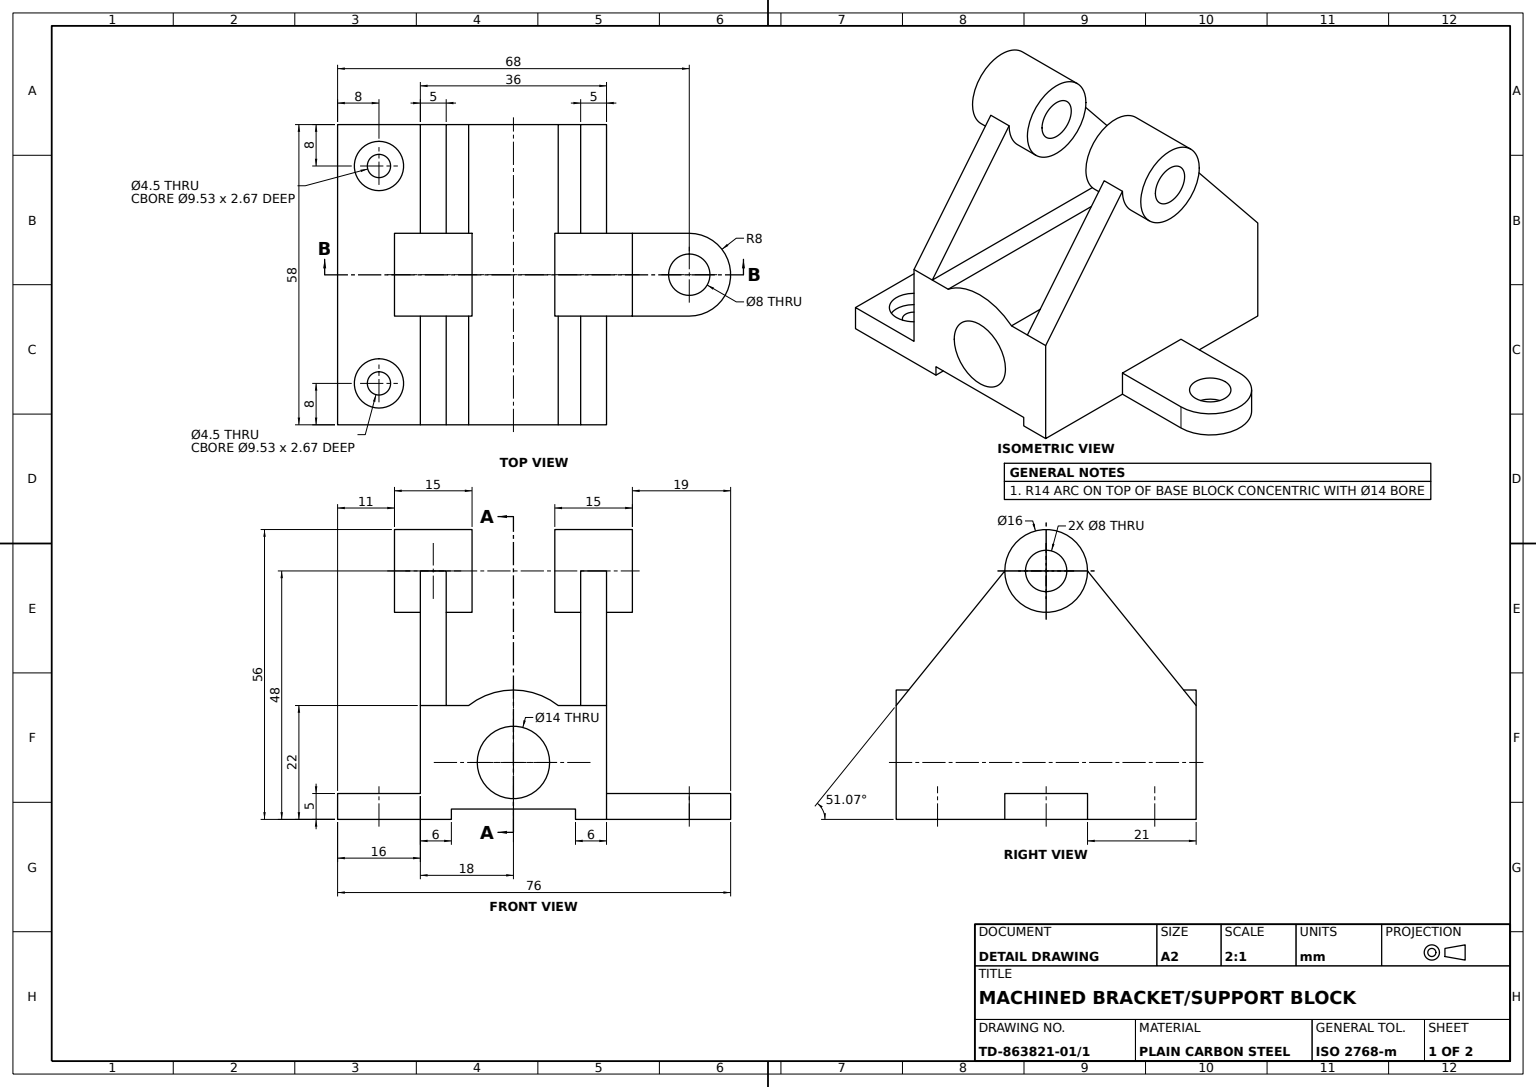
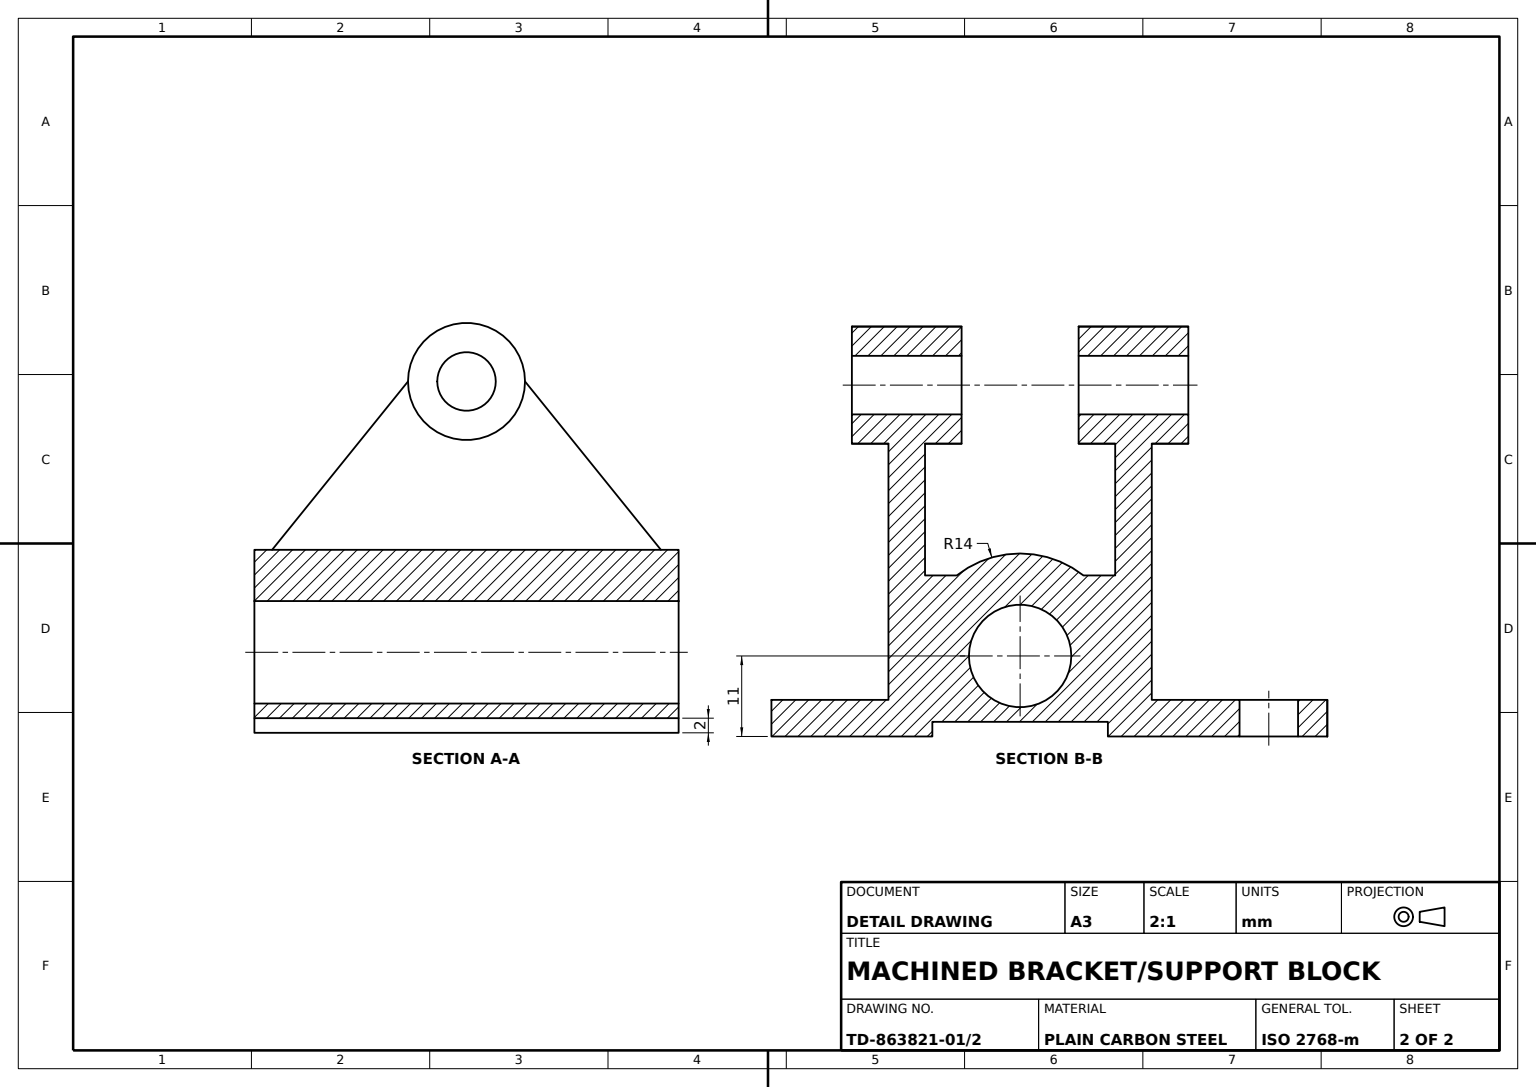
SolidWorks part; units mm, degrees
material "Plain Carbon Steel"
ref_plane "Front Plane" through (0, 0, 0) normal (0, 0, 1) x (1, 0, 0)
ref_plane "Top Plane" through (0, 0, 0) normal (0, 1, 0) x (1, 0, 0)
ref_plane "Right Plane" through (0, 0, 0) normal (1, 0, 0) x (0, 0, -1)
sketch "Base Block Profile" plane through (0, 0, 0) normal (0, 0, 1) x (1, 0, 0)
  line L0 (0, 0) -> (6, 0)
  line L1 (6, 0) -> (6, 2)
  line L2 (6, 2) -> (30, 2)
  line L3 (30, 2) -> (30, 0)
  line L4 (30, 0) -> (36, 0)
  line L5 (36, 0) -> (36, 22)
  line L6 (36, 22) -> (0, 22)
  line L7 (0, 22) -> (0, 0)
  dimension "D1" = 6
  dimension "D2" = 6
  dimension "D3" = 36
  dimension "D4" = 22
  dimension "D5" = 2
extrude "Base Block" add sketch "Base Block Profile" along normal blind 58
sketch "Front Bore Boss Sketch" plane through (0, 0, 58) normal (0, 0, 1) x (1, 0, 0)
  line L0 (4, 11) -> (32, 11)
  line L1 (0, 22) -> (0, 0) construction
  line L2 (0, 0) -> (6, 0) construction
  arc A0 (32, 11) -> (4, 11) centre (18, 11) ccw
  dimension "D1" = 28
  dimension "D2" = 18
  dimension "D3" = 11
extrude "Front Bore Boss" add sketch "Front Bore Boss Sketch" against normal through all
sketch "Front Bore Sketch" plane through (0, 0, 58) normal (0, 0, 1) x (1, 0, 0)
  circle A0 centre (18, 11) radius 7
  dimension "D1" = 14
extrude "Front Bore" cut sketch "Front Bore Sketch" against normal through all
ref_plane "Left Arm Plane" through (0, 0, 0) normal (1, 0, 0) x (0, 0, -1)
sketch "Left Arm Sketch" plane through (0, 0, 0) normal (1, 0, 0) x (0, 0, -1)
  line L0 (-58, 0) -> (0, 0) construction
  circle A0 centre (-29, 48) radius 4
  circle A1 centre (-29, 48) radius 8
  dimension "D1" = 8
  dimension "D2" = 16
  dimension "D3" = 48
  dimension "D4" = 29
extrude "Left Arm" add sketch "Left Arm Sketch" along normal mid plane 10 separate body
sketch "Left Arm Web Sketch" plane through (0, 0, 0) normal (1, 0, 0) x (0, 0, -1)
  line L0 (-21, 48) -> (0, 22)
  line L1 (0, 22) -> (0, 0) construction
  line L2 (-58, 22) -> (0, 22) construction
  line L3 (0, 22) -> (-58, 22)
  line L4 (-58, 22) -> (-37, 48)
  circle A0 centre (-29, 48) radius 8 construction
  arc A1 (-21, 48) -> (-37, 48) centre (-29, 48) cw
extrude "Left Arm Web" add sketch "Left Arm Web Sketch" along normal blind 5
sketch "Left Pivot Boss Sketch" plane through (5, 0, 0) normal (1, 0, 0) x (0, 0, -1)
  circle A0 centre (-29, 48) radius 8
  dimension "D1" = 16
extrude "Left Pivot Boss" add sketch "Left Pivot Boss Sketch" along normal blind 5
sketch "Left Pivot Hole Sketch" plane through (10, 0, 0) normal (1, 0, 0) x (0, 0, -1)
  circle A0 centre (-29, 48) radius 4
  dimension "D1" = 8
extrude "Left Pivot Hole" cut sketch "Left Pivot Hole Sketch" against normal through all
ref_plane "Right Arm Plane" through (36, 0, 0) normal (1, 0, 0) x (0, 0, -1)
sketch "Right Arm Sketch" plane through (36, 0, 0) normal (1, 0, 0) x (0, 0, -1)
  circle A0 centre (-29, 48) radius 4
  circle A1 centre (-29, 48) radius 8
  dimension "D1" = 8
  dimension "D2" = 16
extrude "Right Arm" add sketch "Right Arm Sketch" along normal mid plane 10 separate body
sketch "Right Arm Web Sketch" plane through (36, 0, 0) normal (1, 0, 0) x (0, 0, -1)
  line L0 (-37, 48) -> (-58, 22)
  line L1 (-58, 22) -> (0, 22)
  line L2 (0, 22) -> (-21, 48)
  circle A0 centre (-29, 48) radius 8 construction
  arc A1 (-37, 48) -> (-21, 48) centre (-29, 48) ccw construction
  arc A2 (-37, 48) -> (-21, 48) centre (-29, 48) ccw
extrude "Right Arm Web" add sketch "Right Arm Web Sketch" against normal blind 5
sketch "Right Pivot Boss Sketch" plane through (31, 0, 0) normal (-1, 0, 0) x (0, 0, 1)
  circle A0 centre (29, 48) radius 8
  dimension "D1" = 16
extrude "Right Pivot Boss" add sketch "Right Pivot Boss Sketch" along normal blind 5
sketch "Right Pivot Hole Ø8 Sketch" plane through (26, 0, 0) normal (-1, 0, 0) x (0, 0, 1)
  circle A0 centre (29, 48) radius 4
  dimension "D1" = 8
extrude "Right Pivot Hole Ø8" cut sketch "Right Pivot Hole Ø8 Sketch" against normal through all
ref_plane "Side Lug Plane" through (0, 0, 0) normal (0, 1, 0) x (1, 0, 0)
sketch "Side Lug Sketch" plane through (0, 0, 0) normal (0, 1, 0) x (1, 0, 0)
  line L0 (52, -21) -> (36, -21)
  line L1 (52, -37) -> (36, -37)
  line L2 (36, -37) -> (36, -21)
  line L3 (36, -58) -> (36, 0) construction
  circle A0 centre (52, -29) radius 4
  arc A1 (52, -37) -> (52, -21) centre (52, -29) ccw
  dimension "D1" = 8
  dimension "D2" = 16
  dimension "D3" = 16
extrude "Side Lug" add sketch "Side Lug Sketch" along normal blind 5
ref_plane "Mounting Tab Plane" through (0, 0, 0) normal (0, 1, 0) x (1, 0, 0)
sketch "Mounting Tab Sketch" plane through (0, 0, 0) normal (0, 1, 0) x (1, 0, 0)
  line L0 (0, 0) -> (-16, 0)
  line L1 (-16, 0) -> (-16, -58)
  line L2 (-16, -58) -> (0, -58)
  line L3 (0, -58) -> (0, 0)
  dimension "D1" = 16
extrude "Mounting Tab" add sketch "Mounting Tab Sketch" along normal blind 5
hole_wizard "M5 Counterbore Hole" positions "Sketch43" profile "Sketch44" counterbore size "M5" standard "ISO" end condition through all
sketch "Sketch43" plane through (0, 5, 0) normal (0, 1, 0) x (1, 0, 0)
  line L0 (0, 0) -> (-16, 0) construction
  line L1 (-16, 0) -> (-16, -58) construction
  line L2 (-16, -58) -> (0, -58) construction
  point P0 (-8, -8)
  point P2 (-8, -50)
  dimension "D1" = 8
  dimension "D2" = 8
  dimension "D3" = 8
  dimension "D4" = 8
sketch "Sketch44" plane through (-8, 5, 8) normal (1, 0, 0) x (0, 0, 1)
  line L0 (0, 0) -> (0, 5)
  line L1 (0, 5) -> (2.25, 5)
  line L3 (2.25, 5) -> (2.25, 2.67)
  line L4 (2.25, 2.67) -> (4.765, 2.67)
  line L5 (4.765, 2.67) -> (4.765, 0)
  line L7 (4.765, 0) -> (0, 0)
  line L11 (0, -6.35) -> (0, 107.95) construction
  dimension "Thru Hole Dia." = 4.5
  dimension "Thru Hole Depth" = 5
  dimension "C'Bore Dia." = 9.53
  dimension "C'Bore Depth" = 2.67
